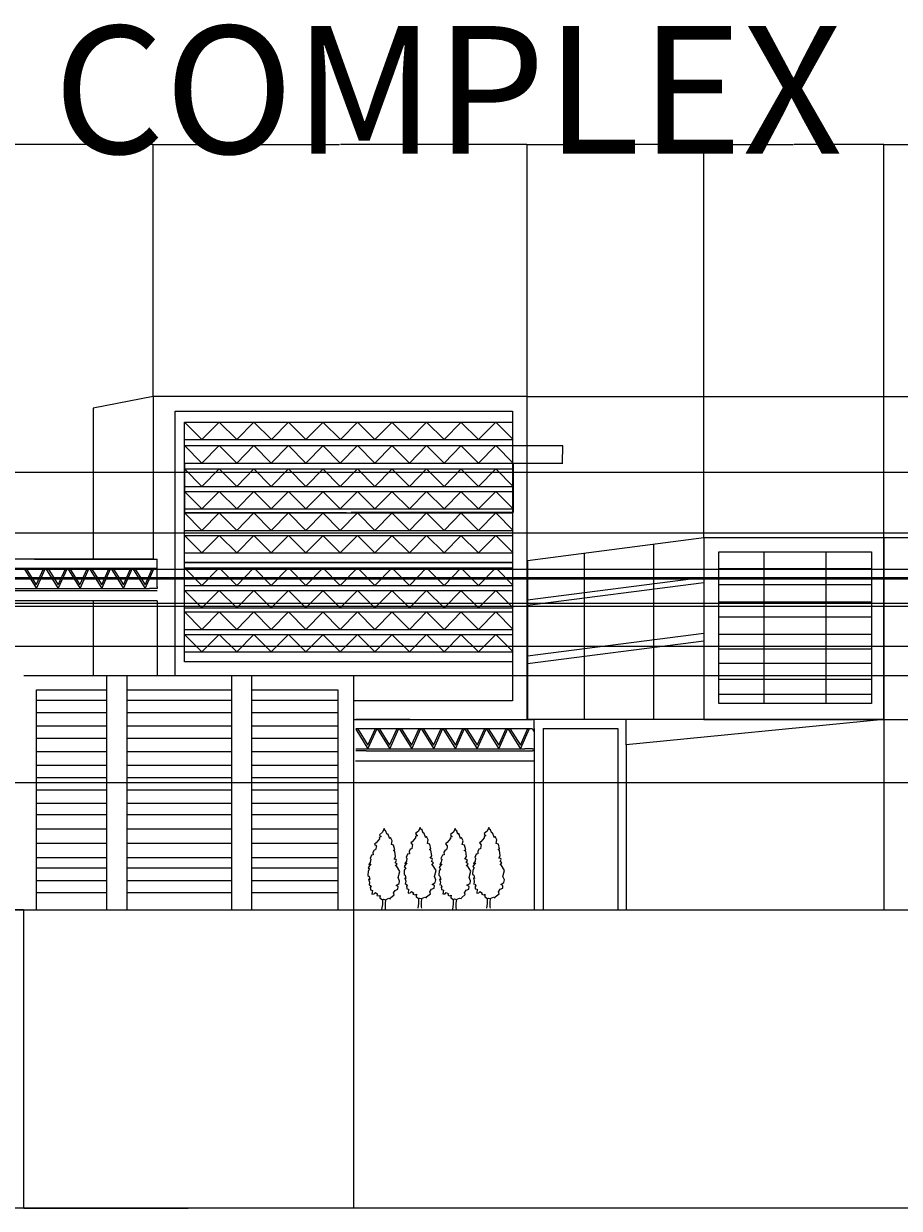
# Model space of a CAD drawing. Units: inches. Extents: x -2248 to 2617, y -128 to 922.
# Tile 6 of 7: x 820 to 1596, y -128 to 922. Entities that reach past the tile are written whole.
import ezdxf

# ---------------------------------------------------------------- set-up
doc = ezdxf.new("R2010")
doc.units = ezdxf.units.IN
doc.header["$MEASUREMENT"] = 0
for name, color, linetype, lineweight in [('A-ANNO-DIMS', 2, 'Continuous', 18), ('A-ANNO-TEXT', 7, 'Continuous', 25), ('A-ELEV', 7, 'Continuous', 25), ('A-ELEV-FACD', 8, 'Continuous', 13), ('L-PLNT', 3, 'Continuous', 18)]:
    doc.layers.add(name, color=color, linetype=linetype, lineweight=lineweight)
doc.styles.get("Standard").update_dxf_attribs({"font": 'arial.ttf'})
doc.dimstyles.get("Standard").update_dxf_attribs({"dimtxt": 0.18, "dimasz": 0.18, "dimexe": 0.18, "dimexo": 0.0625, "dimgap": 0.09, "dimtad": 0, "dimtih": 1, "dimtoh": 1, "dimdec": 4, "dimzin": 0, "dimdsep": 46, "dimtxsty": 'Standard', "dimcen": 0.09, "dimadec": 0, "dimazin": 0, "dimtfac": 1, "dimtdec": 4, "dimtofl": 0, "dimtmove": 0, "dimatfit": 3, "dimfxl": 1, "dimtolj": 1, "dimtzin": 0, "dimarcsym": 0})

# ---------------------------------------------------------------- blocks, each defined once
blk = doc.blocks.new('*U3')
blk.add_lwpolyline([(-2.754, 191.699), (-6.78, 182.851), (-13.682, 176.953), (-11.956, 173.266), (-9.656, 172.529), (-14.257, 170.317), (-13.682, 167.368), (-21.733, 157.783), (-25.184, 154.834), (-21.158, 150.41), (-21.733, 147.461), (-22.884, 140.825), (-26.334, 140.087), (-29.21, 134.926), (-28.635, 129.028), (-32.661, 128.291), (-36.111, 120.18), (-34.386, 118.706), (-35.536, 111.333), (-38.987, 106.171), (-34.386, 107.646), (-40.712, 98.798), (-37.261, 95.849), (-40.712, 90.688), (-41.287, 80.366), (-38.412, 78.154), (-36.686, 70.781), (-39.562, 71.518), (-37.261, 64.145), (-38.412, 57.509), (-36.111, 58.247), (-33.236, 52.348), (-35.536, 53.086), (-34.961, 46.45), (-30.36, 44.975), (-31.51, 36.128), (-26.334, 36.865), (-23.459, 39.814), (-18.283, 36.128), (-20.008, 33.178), (-14.832, 31.704), (-11.956, 33.178), (-12.531, 27.28), (-6.205, 22.856), (-3.905, 24.331), (0.121, 22.856), (8.173, 26.543), (11.624, 25.068), (12.199, 27.28), (21.4, 34.653), (19.675, 39.077), (23.701, 44.975), (30.027, 47.924), (30.602, 53.823), (25.426, 56.772), (32.903, 61.196), (34.053, 67.094), (30.602, 75.205), (34.628, 89.951), (26.576, 103.222), (23.701, 103.222), (28.302, 107.646), (23.701, 110.595), (26.576, 115.756), (25.426, 117.968), (20.825, 118.706), (24.276, 124.604), (22.551, 137.876), (19.1, 139.35), (22.551, 140.825), (19.675, 151.884), (14.499, 153.359), (16.224, 162.207), (12.199, 170.317), (10.473, 167.368), (5.872, 179.165), (4.147, 177.69), (0.696, 187.275), (-0.454, 185.8)], close=True)
for points in [[(-6.813, 23.669), (-6.813, 11.669), (-8.627, 0)], [(0.387, 23.669), (-0.576, 13.271), (-0.576, 3.686), (0, 0)]]:
    blk.add_lwpolyline(points)
blk = doc.blocks.new('FACADE-SCREEN-PANEL')
for p, q in [((0, 15.5), (290.7, 15.5)), ((0, 15.5), (15.6, 0)), ((15.6, 0), (30.8, 15.5)), ((30.8, 15.5), (46.4, 0)), ((46.4, 0), (61.6, 15.5)), ((61.5, 15.5), (77, 0)), ((77, 0), (92.2, 15.5)), ((92.1, 15.5), (107.7, 0)), ((107.7, 0), (122.9, 15.5)), ((122.6, 15.5), (138.1, 0)), ((138.1, 0), (153.4, 15.5)), ((153.2, 15.5), (168.8, 0)), ((168.8, 0), (184, 15.5)), ((183.8, 15.5), (199.3, 0)), ((199.3, 0), (214.5, 15.5)), ((214.4, 15.5), (230, 0)), ((230, 0), (245.2, 15.5)), ((245, 15.5), (260.5, 0)), ((260.5, 0), (275.8, 15.5)), ((275.8, 15.5), (291.3, 0)), ((0, 0), (291.3, 0))]:
    blk.add_line(p, q)
blk = doc.blocks.new('*D10')
at = {"layer": 'A-ANNO-DIMS', "color": 0, "lineweight": -2, "transparency": 16777216}
for p, q in [((962.6, 532.4), (962.6, 488.5)), ((1253.9, 532.4), (1253.9, 488.5)), ((962.8, 488.7), (1106.1, 488.7)), ((1253.7, 488.7), (1110.4, 488.7))]:
    blk.add_line(p, q, dxfattribs=at)
at = {"layer": 'A-ANNO-DIMS', "color": 0, "transparency": 16777216}
for points in [[(962.8, 488.7), (962.8, 488.7), (962.6, 488.7)], [(1253.7, 488.7), (1253.7, 488.7), (1253.9, 488.7)]]:
    blk.add_solid(points, dxfattribs=at)
at = {"layer": 'Defpoints', "color": 0, "transparency": 16777216}
for p in [(962.6, 532.4), (1253.9, 532.4), (1253.9, 488.7)]:
    blk.add_point(p, dxfattribs=at)
at = {"layer": 'A-ANNO-DIMS', "color": 0, "transparency": 16777216, "insert": (1108.3, 488.7), "char_height": 0.18, "attachment_point": 5}
blk.add_mtext('\\A1;FACADE SCREEN PANEL 291 TYP.', dxfattribs=at)
blk = doc.blocks.new('*D11')
at = {"layer": 'A-ANNO-DIMS', "color": 0, "lineweight": -2, "transparency": 16777216}
for p, q in [((1254, 547.9), (1297.8, 547.9)), ((1297.6, 547.7), (1297.6, 540.3)), ((1297.6, 532.6), (1297.6, 540)), ((1254, 532.4), (1297.8, 532.4))]:
    blk.add_line(p, q, dxfattribs=at)
at = {"layer": 'A-ANNO-DIMS', "color": 0, "transparency": 16777216}
for points in [[(1297.6, 547.7), (1297.7, 547.7), (1297.6, 547.9)], [(1297.6, 532.6), (1297.7, 532.6), (1297.6, 532.4)]]:
    blk.add_solid(points, dxfattribs=at)
at = {"layer": 'Defpoints', "color": 0, "transparency": 16777216}
for p in [(1253.9, 547.9), (1297.6, 547.9), (1253.9, 532.4)]:
    blk.add_point(p, dxfattribs=at)
at = {"layer": 'A-ANNO-DIMS', "color": 0, "transparency": 16777216, "insert": (1297.6, 540.1), "char_height": 0.18, "attachment_point": 5}
blk.add_mtext('\\A1;15 TYP.', dxfattribs=at)
blk = doc.blocks.new('*D16')
at = {"layer": 'A-ANNO-DIMS', "color": 0, "lineweight": -2, "transparency": 16777216}
for p, q in [((45.9, 438.4), (2616.5, 438.4)), ((2616.3, 438.3), (2616.3, 287.6)), ((2616.3, 136.6), (2616.3, 287.3)), ((45.9, 136.5), (2616.5, 136.5))]:
    blk.add_line(p, q, dxfattribs=at)
at = {"layer": 'A-ANNO-DIMS', "color": 0, "transparency": 16777216}
for points in [[(2616.2, 438.3), (2616.3, 438.3), (2616.3, 438.4)], [(2616.2, 136.6), (2616.3, 136.6), (2616.3, 136.5)]]:
    blk.add_solid(points, dxfattribs=at)
at = {"layer": 'Defpoints', "color": 0, "transparency": 16777216}
for p in [(45.8, 438.4), (45.8, 136.5), (2616.3, 136.5)]:
    blk.add_point(p, dxfattribs=at)
at = {"layer": 'A-ANNO-DIMS', "color": 0, "transparency": 16777216, "insert": (2616.3, 287.4), "char_height": 0.18, "attachment_point": 5}
blk.add_mtext('\\A1;302', dxfattribs=at)
blk = doc.blocks.new('*D17')
at = {"layer": 'A-ANNO-DIMS', "color": 0, "lineweight": -2, "transparency": 16777216}
for p, q in [((625.1, 524.3), (2616.5, 524.3)), ((2616.3, 524.1), (2616.3, 330.6)), ((2616.3, 136.6), (2616.3, 330.2)), ((553.6, 136.5), (2616.5, 136.5))]:
    blk.add_line(p, q, dxfattribs=at)
at = {"layer": 'A-ANNO-DIMS', "color": 0, "transparency": 16777216}
for points in [[(2616.2, 524.1), (2616.3, 524.1), (2616.3, 524.3)], [(2616.2, 136.6), (2616.3, 136.6), (2616.3, 136.5)]]:
    blk.add_solid(points, dxfattribs=at)
at = {"layer": 'Defpoints', "color": 0, "transparency": 16777216}
for p in [(625.1, 524.3), (553.6, 136.5), (2616.3, 136.5)]:
    blk.add_point(p, dxfattribs=at)
at = {"layer": 'A-ANNO-DIMS', "color": 0, "transparency": 16777216, "insert": (2616.3, 330.4), "char_height": 0.18, "attachment_point": 5}
blk.add_mtext('\\A1;387.9', dxfattribs=at)
blk = doc.blocks.new('*D20')
at = {"layer": 'A-ANNO-DIMS', "color": 0, "lineweight": -2, "transparency": 16777216}
for p, q in [((-1595.3, 429.9), (2616.5, 429.9)), ((2616.3, 429.7), (2616.3, 417.9)), ((2616.3, 405.8), (2616.3, 417.5)), ((-1653.9, 405.6), (2616.5, 405.6))]:
    blk.add_line(p, q, dxfattribs=at)
at = {"layer": 'A-ANNO-DIMS', "color": 0, "transparency": 16777216}
for points in [[(2616.2, 429.7), (2616.3, 429.7), (2616.3, 429.9)], [(2616.2, 405.8), (2616.3, 405.8), (2616.3, 405.6)]]:
    blk.add_solid(points, dxfattribs=at)
at = {"layer": 'Defpoints', "color": 0, "transparency": 16777216}
for p in [(-1595.4, 429.9), (-1654, 405.6), (2616.3, 405.6)]:
    blk.add_point(p, dxfattribs=at)
at = {"layer": 'A-ANNO-DIMS', "color": 0, "transparency": 16777216, "insert": (2616.3, 417.7), "char_height": 0.18, "attachment_point": 5}
blk.add_mtext('\\A1;24.3', dxfattribs=at)
blk = doc.blocks.new('*D21')
at = {"layer": 'A-ANNO-DIMS', "color": 0, "lineweight": -2, "transparency": 16777216}
for p, q in [((-1125.3, 470.6), (2616.5, 470.6)), ((2616.3, 470.4), (2616.3, 451)), ((2616.3, 431.1), (2616.3, 450.6)), ((-1257.9, 430.9), (2616.5, 430.9))]:
    blk.add_line(p, q, dxfattribs=at)
at = {"layer": 'A-ANNO-DIMS', "color": 0, "transparency": 16777216}
for points in [[(2616.2, 470.4), (2616.3, 470.4), (2616.3, 470.6)], [(2616.2, 431.1), (2616.3, 431.1), (2616.3, 430.9)]]:
    blk.add_solid(points, dxfattribs=at)
at = {"layer": 'Defpoints', "color": 0, "transparency": 16777216}
for p in [(-1125.4, 470.6), (-1258, 430.9), (2616.3, 430.9)]:
    blk.add_point(p, dxfattribs=at)
at = {"layer": 'A-ANNO-DIMS', "color": 0, "transparency": 16777216, "insert": (2616.3, 450.8), "char_height": 0.18, "attachment_point": 5}
blk.add_mtext('\\A1;39.705', dxfattribs=at)
blk = doc.blocks.new('*D22')
at = {"layer": 'A-ANNO-DIMS', "color": 0, "lineweight": -2, "transparency": 16777216}
for p, q in [((-733.3, 408.4), (2616.5, 408.4)), ((2616.3, 408.2), (2616.3, 329.1)), ((2616.3, 249.6), (2616.3, 328.7)), ((-719.1, 249.4), (2616.5, 249.4))]:
    blk.add_line(p, q, dxfattribs=at)
at = {"layer": 'A-ANNO-DIMS', "color": 0, "transparency": 16777216}
for points in [[(2616.2, 408.2), (2616.3, 408.2), (2616.3, 408.4)], [(2616.2, 249.6), (2616.3, 249.6), (2616.3, 249.4)]]:
    blk.add_solid(points, dxfattribs=at)
at = {"layer": 'Defpoints', "color": 0, "transparency": 16777216}
for p in [(-733.4, 408.4), (-719.2, 249.4), (2616.3, 249.4)]:
    blk.add_point(p, dxfattribs=at)
at = {"layer": 'A-ANNO-DIMS', "color": 0, "transparency": 16777216, "insert": (2616.3, 328.9), "char_height": 0.18, "attachment_point": 5}
blk.add_mtext('\\A1;159.02', dxfattribs=at)
blk = doc.blocks.new('*D23')
at = {"layer": 'A-ANNO-DIMS', "color": 0, "lineweight": -2, "transparency": 16777216}
for p, q in [((-719.1, 249.4), (2616.5, 249.4)), ((2616.3, 249.2), (2616.3, 193.1)), ((2616.3, 136.6), (2616.3, 192.7)), ((-719.1, 136.5), (2616.5, 136.5))]:
    blk.add_line(p, q, dxfattribs=at)
at = {"layer": 'A-ANNO-DIMS', "color": 0, "transparency": 16777216}
for points in [[(2616.2, 249.2), (2616.3, 249.2), (2616.3, 249.4)], [(2616.2, 136.6), (2616.3, 136.6), (2616.3, 136.5)]]:
    blk.add_solid(points, dxfattribs=at)
at = {"layer": 'Defpoints', "color": 0, "transparency": 16777216}
for p in [(-719.2, 249.4), (-719.2, 136.5), (2616.3, 136.5)]:
    blk.add_point(p, dxfattribs=at)
at = {"layer": 'A-ANNO-DIMS', "color": 0, "transparency": 16777216, "insert": (2616.3, 192.9), "char_height": 0.18, "attachment_point": 5}
blk.add_mtext('\\A1;112.94', dxfattribs=at)
blk = doc.blocks.new('*D24')
at = {"layer": 'A-ANNO-DIMS', "color": 0, "lineweight": -2, "transparency": 16777216}
for p, q in [((-316.1, 370.3), (2616.5, 370.3)), ((2616.3, 370.1), (2616.3, 253.6)), ((2616.3, 136.6), (2616.3, 253.2)), ((-159.8, 136.5), (2616.5, 136.5))]:
    blk.add_line(p, q, dxfattribs=at)
at = {"layer": 'A-ANNO-DIMS', "color": 0, "transparency": 16777216}
for points in [[(2616.2, 370.1), (2616.3, 370.1), (2616.3, 370.3)], [(2616.2, 136.6), (2616.3, 136.6), (2616.3, 136.5)]]:
    blk.add_solid(points, dxfattribs=at)
at = {"layer": 'Defpoints', "color": 0, "transparency": 16777216}
for p in [(-316.2, 370.3), (-159.9, 136.5), (2616.3, 136.5)]:
    blk.add_point(p, dxfattribs=at)
at = {"layer": 'A-ANNO-DIMS', "color": 0, "transparency": 16777216, "insert": (2616.3, 253.4), "char_height": 0.18, "attachment_point": 5}
blk.add_mtext('\\A1;233.87', dxfattribs=at)
blk = doc.blocks.new('*D25')
at = {"layer": 'A-ANNO-DIMS', "color": 0, "lineweight": -2, "transparency": 16777216}
for p, q in [((1112.5, 344.2), (2616.5, 344.2)), ((2616.3, 344), (2616.3, 240.5)), ((2616.3, 136.6), (2616.3, 240.2)), ((1112.5, 136.5), (2616.5, 136.5))]:
    blk.add_line(p, q, dxfattribs=at)
at = {"layer": 'A-ANNO-DIMS', "color": 0, "transparency": 16777216}
for points in [[(2616.2, 344), (2616.3, 344), (2616.3, 344.2)], [(2616.2, 136.6), (2616.3, 136.6), (2616.3, 136.5)]]:
    blk.add_solid(points, dxfattribs=at)
at = {"layer": 'Defpoints', "color": 0, "transparency": 16777216}
for p in [(1112.5, 344.2), (1112.5, 136.5), (2616.3, 136.5)]:
    blk.add_point(p, dxfattribs=at)
at = {"layer": 'A-ANNO-DIMS', "color": 0, "transparency": 16777216, "insert": (2616.3, 240.3), "char_height": 0.18, "attachment_point": 5}
blk.add_mtext('\\A1;207.78', dxfattribs=at)
blk = doc.blocks.new('*D26')
at = {"layer": 'A-ANNO-DIMS', "color": 0, "lineweight": -2, "transparency": 16777216}
for p, q in [((1582.3, 466.3), (2616.5, 466.3)), ((2616.3, 466.1), (2616.3, 385.9)), ((2616.3, 305.4), (2616.3, 385.6)), ((1582.3, 305.2), (2616.5, 305.2))]:
    blk.add_line(p, q, dxfattribs=at)
at = {"layer": 'A-ANNO-DIMS', "color": 0, "transparency": 16777216}
for points in [[(2616.2, 466.1), (2616.3, 466.1), (2616.3, 466.3)], [(2616.2, 305.4), (2616.3, 305.4), (2616.3, 305.2)]]:
    blk.add_solid(points, dxfattribs=at)
at = {"layer": 'Defpoints', "color": 0, "transparency": 16777216}
for p in [(1582.2, 466.3), (1582.2, 305.2), (2616.3, 305.2)]:
    blk.add_point(p, dxfattribs=at)
at = {"layer": 'A-ANNO-DIMS', "color": 0, "transparency": 16777216, "insert": (2616.3, 385.8), "char_height": 0.18, "attachment_point": 5}
blk.add_mtext('\\A1;161.04', dxfattribs=at)
blk = doc.blocks.new('*D28')
at = {"layer": 'A-ANNO-DIMS', "color": 0, "lineweight": -2, "transparency": 16777216}
for p, q in [((1266.1, 591.3), (2616.5, 591.3)), ((2616.3, 591.1), (2616.3, 364)), ((2616.3, 136.6), (2616.3, 363.7)), ((2058.4, 136.5), (2616.5, 136.5))]:
    blk.add_line(p, q, dxfattribs=at)
at = {"layer": 'A-ANNO-DIMS', "color": 0, "transparency": 16777216}
for points in [[(2616.2, 591.1), (2616.3, 591.1), (2616.3, 591.3)], [(2616.2, 136.6), (2616.3, 136.6), (2616.3, 136.5)]]:
    blk.add_solid(points, dxfattribs=at)
at = {"layer": 'Defpoints', "color": 0, "transparency": 16777216}
for p in [(1266.1, 591.3), (2616.3, 591.3), (2058.4, 136.5)]:
    blk.add_point(p, dxfattribs=at)
at = {"layer": 'A-ANNO-DIMS', "color": 0, "transparency": 16777216, "insert": (2616.3, 363.9), "char_height": 0.18, "attachment_point": 5}
blk.add_mtext('\\A1;454.8', dxfattribs=at)
blk = doc.blocks.new('*D31')
at = {"layer": 'A-ANNO-DIMS', "color": 0, "lineweight": -2, "transparency": 16777216}
for p, q in [((934.8, 447.2), (-2247.7, 447.2)), ((-2247.5, 447), (-2247.5, 292)), ((-2247.5, 136.6), (-2247.5, 291.6)), ((820, 136.5), (-2247.7, 136.5))]:
    blk.add_line(p, q, dxfattribs=at)
at = {"layer": 'A-ANNO-DIMS', "color": 0, "transparency": 16777216}
for points in [[(-2247.5, 447), (-2247.5, 447), (-2247.5, 447.2)], [(-2247.5, 136.6), (-2247.5, 136.6), (-2247.5, 136.5)]]:
    blk.add_solid(points, dxfattribs=at)
at = {"layer": 'Defpoints', "color": 0, "transparency": 16777216}
for p in [(934.9, 447.2), (-2247.5, 136.5), (820.1, 136.5)]:
    blk.add_point(p, dxfattribs=at)
at = {"layer": 'A-ANNO-DIMS', "color": 0, "transparency": 16777216, "insert": (-2247.5, 291.8), "char_height": 0.18, "attachment_point": 5}
blk.add_mtext('\\A1;310.7', dxfattribs=at)
blk = doc.blocks.new('*D33')
at = {"layer": 'A-ANNO-DIMS', "color": 0, "lineweight": -2, "transparency": 16777216}
for p, q in [((2393, 136.4), (2393, -127.9)), ((-2024.3, 122), (-2024.3, -127.9)), ((-2024.1, -127.7), (184, -127.7)), ((2392.8, -127.7), (184.7, -127.7))]:
    blk.add_line(p, q, dxfattribs=at)
at = {"layer": 'A-ANNO-DIMS', "color": 0, "transparency": 16777216}
for points in [[(-2024.1, -127.6), (-2024.1, -127.7), (-2024.3, -127.7)], [(2392.8, -127.6), (2392.8, -127.7), (2393, -127.7)]]:
    blk.add_solid(points, dxfattribs=at)
at = {"layer": 'Defpoints', "color": 0, "transparency": 16777216}
for p in [(2393, 136.5), (-2024.3, 122.1), (2393, -127.7)]:
    blk.add_point(p, dxfattribs=at)
at = {"layer": 'A-ANNO-DIMS', "color": 0, "transparency": 16777216, "insert": (184.4, -127.7), "char_height": 0.18, "attachment_point": 5}
blk.add_mtext('\\A1;4417', dxfattribs=at)
blk = doc.blocks.new('*D50')
at = {"layer": 'A-ANNO-DIMS', "color": 0, "lineweight": -2, "transparency": 16777216}
for p, q in [((625.1, 524.4), (625.1, 814.7)), ((625.2, 814.5), (779.6, 814.5)), ((934.7, 814.5), (780.4, 814.5)), ((934.9, 591.3), (934.9, 814.7))]:
    blk.add_line(p, q, dxfattribs=at)
at = {"layer": 'A-ANNO-DIMS', "color": 0, "transparency": 16777216}
for points in [[(625.2, 814.5), (625.2, 814.5), (625.1, 814.5)], [(934.7, 814.5), (934.7, 814.5), (934.9, 814.5)]]:
    blk.add_solid(points, dxfattribs=at)
at = {"layer": 'Defpoints', "color": 0, "transparency": 16777216}
for p in [(934.9, 814.5), (934.9, 591.3), (625.1, 524.3)]:
    blk.add_point(p, dxfattribs=at)
at = {"layer": 'A-ANNO-DIMS', "color": 0, "transparency": 16777216, "insert": (780, 814.5), "char_height": 0.18, "attachment_point": 5}
blk.add_mtext('\\A1;309.8', dxfattribs=at)
blk = doc.blocks.new('*D51')
at = {"layer": 'A-ANNO-DIMS', "color": 0, "lineweight": -2, "transparency": 16777216}
for p, q in [((934.9, 591.3), (934.9, 814.7)), ((935, 814.5), (1100.1, 814.5)), ((1265.9, 814.5), (1100.9, 814.5)), ((1266.1, 591.3), (1266.1, 814.7))]:
    blk.add_line(p, q, dxfattribs=at)
at = {"layer": 'A-ANNO-DIMS', "color": 0, "transparency": 16777216}
for points in [[(935, 814.5), (935, 814.5), (934.9, 814.5)], [(1265.9, 814.5), (1265.9, 814.5), (1266.1, 814.5)]]:
    blk.add_solid(points, dxfattribs=at)
at = {"layer": 'Defpoints', "color": 0, "transparency": 16777216}
for p in [(1266.1, 814.5), (934.9, 591.3), (1266.1, 591.3)]:
    blk.add_point(p, dxfattribs=at)
at = {"layer": 'A-ANNO-DIMS', "color": 0, "transparency": 16777216, "insert": (1100.5, 814.5), "char_height": 0.18, "attachment_point": 5}
blk.add_mtext('\\A1;331.2', dxfattribs=at)
blk = doc.blocks.new('*D52')
at = {"layer": 'A-ANNO-DIMS', "color": 0, "lineweight": -2, "transparency": 16777216}
for p, q in [((1266.1, 591.3), (1266.1, 814.7)), ((1266.3, 814.5), (1343.9, 814.5)), ((1422.5, 814.5), (1344.8, 814.5)), ((1422.7, 466.3), (1422.7, 814.7))]:
    blk.add_line(p, q, dxfattribs=at)
at = {"layer": 'A-ANNO-DIMS', "color": 0, "transparency": 16777216}
for points in [[(1266.3, 814.5), (1266.3, 814.5), (1266.1, 814.5)], [(1422.5, 814.5), (1422.5, 814.5), (1422.7, 814.5)]]:
    blk.add_solid(points, dxfattribs=at)
at = {"layer": 'Defpoints', "color": 0, "transparency": 16777216}
for p in [(1422.7, 814.5), (1266.1, 591.3), (1422.7, 466.3)]:
    blk.add_point(p, dxfattribs=at)
at = {"layer": 'A-ANNO-DIMS', "color": 0, "transparency": 16777216, "insert": (1344.4, 814.5), "char_height": 0.18, "attachment_point": 5}
blk.add_mtext('\\A1;156.62', dxfattribs=at)
blk = doc.blocks.new('*D53')
at = {"layer": 'A-ANNO-DIMS', "color": 0, "lineweight": -2, "transparency": 16777216}
for p, q in [((1422.7, 466.3), (1422.7, 814.7)), ((1422.9, 814.5), (1502.1, 814.5)), ((1582, 814.5), (1502.8, 814.5)), ((1582.2, 466.3), (1582.2, 814.7))]:
    blk.add_line(p, q, dxfattribs=at)
at = {"layer": 'A-ANNO-DIMS', "color": 0, "transparency": 16777216}
for points in [[(1422.9, 814.5), (1422.9, 814.5), (1422.7, 814.5)], [(1582, 814.5), (1582, 814.5), (1582.2, 814.5)]]:
    blk.add_solid(points, dxfattribs=at)
at = {"layer": 'Defpoints', "color": 0, "transparency": 16777216}
for p in [(1582.2, 814.5), (1422.7, 466.3), (1582.2, 466.3)]:
    blk.add_point(p, dxfattribs=at)
at = {"layer": 'A-ANNO-DIMS', "color": 0, "transparency": 16777216, "insert": (1502.5, 814.5), "char_height": 0.18, "attachment_point": 5}
blk.add_mtext('\\A1;159.5', dxfattribs=at)
blk = doc.blocks.new('*D54')
at = {"layer": 'A-ANNO-DIMS', "color": 0, "lineweight": -2, "transparency": 16777216}
for p, q in [((1582.2, 305.3), (1582.2, 814.7)), ((1582.4, 814.5), (1819.8, 814.5)), ((2058.2, 814.5), (1820.7, 814.5)), ((2058.4, 305.3), (2058.4, 814.7))]:
    blk.add_line(p, q, dxfattribs=at)
at = {"layer": 'A-ANNO-DIMS', "color": 0, "transparency": 16777216}
for points in [[(1582.4, 814.5), (1582.4, 814.5), (1582.2, 814.5)], [(2058.2, 814.5), (2058.2, 814.5), (2058.4, 814.5)]]:
    blk.add_solid(points, dxfattribs=at)
at = {"layer": 'Defpoints', "color": 0, "transparency": 16777216}
for p in [(2058.4, 814.5), (1582.2, 305.2), (2058.4, 305.2)]:
    blk.add_point(p, dxfattribs=at)
at = {"layer": 'A-ANNO-DIMS', "color": 0, "transparency": 16777216, "insert": (1820.3, 814.5), "char_height": 0.18, "attachment_point": 5}
blk.add_mtext('\\A1;476.15', dxfattribs=at)
blk = doc.blocks.new('*D57')
at = {"layer": 'A-ANNO-DIMS', "color": 0, "lineweight": -2, "transparency": 16777216}
for p, q in [((820.1, 136.4), (820.1, -127.9)), ((1112.5, 136.4), (1112.5, -127.9)), ((820.3, -127.7), (965.9, -127.7)), ((1112.3, -127.7), (966.7, -127.7))]:
    blk.add_line(p, q, dxfattribs=at)
at = {"layer": 'A-ANNO-DIMS', "color": 0, "transparency": 16777216}
for points in [[(820.3, -127.6), (820.3, -127.7), (820.1, -127.7)], [(1112.3, -127.6), (1112.3, -127.7), (1112.5, -127.7)]]:
    blk.add_solid(points, dxfattribs=at)
at = {"layer": 'Defpoints', "color": 0, "transparency": 16777216}
for p in [(820.1, 136.5), (1112.5, 136.5), (1112.5, -127.7)]:
    blk.add_point(p, dxfattribs=at)
at = {"layer": 'A-ANNO-DIMS', "color": 0, "transparency": 16777216, "insert": (966.3, -127.7), "char_height": 0.18, "attachment_point": 5}
blk.add_mtext('\\A1;292.4', dxfattribs=at)

msp = doc.modelspace()

# ---------------------------------------------------------------- linework, layer by layer
at = {"layer": 'A-ELEV'}
for p, q in [((934.8599, 591.2689), (881.9153, 581.0202)), ((1266.0706, 591.2689), (934.8599, 591.2689)), ((934.8599, 591.2689), (934.8599, 447.1806)), ((1266.0706, 305.2491), (1266.0706, 591.2689)), ((881.9153, 581.0202), (881.9153, 447.1785)), ((954.5101, 578.2931), (1253.2702, 578.2931)), ((954.5101, 344.2299), (954.5101, 578.2931)), ((1253.2702, 578.2931), (1253.2702, 321.5917)), ((962.601, 568.6073), (1253.2702, 568.6073)), ((962.601, 356.3956), (962.601, 568.6073)), ((962.601, 568.6073), (978.1733, 553.154)), ((978.1733, 553.154), (993.3817, 568.6073)), ((993.3845, 568.6073), (1008.9567, 553.154)), ((1008.9567, 553.154), (1024.1652, 568.6073)), ((1024.0616, 568.6073), (1039.6339, 553.154)), ((1039.6339, 553.154), (1054.8423, 568.6073)), ((1054.6964, 568.6073), (1070.2686, 553.154)), ((1070.2686, 553.154), (1085.477, 568.6073)), ((1085.1738, 568.6073), (1100.746, 553.154)), ((1100.746, 553.154), (1115.9544, 568.6073)), ((1115.8362, 568.6073), (1131.4084, 553.154)), ((1131.4084, 553.154), (1146.6169, 568.6073)), ((1146.3674, 568.6073), (1161.9396, 553.154)), ((1161.9396, 553.154), (1177.1481, 568.6073)), ((1177.0447, 568.6073), (1192.617, 553.154)), ((1192.617, 553.154), (1207.8254, 568.6073)), ((1207.576, 568.6073), (1223.1482, 553.154)), ((1223.1482, 553.154), (1238.3566, 568.6073)), ((1238.351, 568.6073), (1253.9233, 553.154)), ((962.601, 553.154), (1253.9233, 553.154)), ((1266.5247, 446.1129), (1422.6951, 466.287)), ((1422.6951, 466.287), (1422.6951, 305.2491)), ((1422.6951, 466.287), (1582.2049, 466.287)), ((1582.2049, 466.287), (1582.2049, 305.2491)), ((1316.8274, 452.611), (1316.8274, 305.2491)), ((1377.9797, 460.5106), (1377.9797, 305.2491)), ((1435.9942, 453.6809), (1571.2541, 453.6809)), ((1436.0053, 319.2369), (1436.0053, 453.6809)), ((1476.1529, 319.2369), (1476.1529, 453.6809)), ((1531.177, 319.2369), (1531.177, 453.6809)), ((1571.2541, 453.6809), (1571.2541, 319.2369)), ((829.7811, 447.1806), (781.9719, 447.1806)), ((829.7811, 447.1806), (938.3811, 447.1806)), ((934.8599, 447.1806), (938.3811, 447.1806)), ((938.3811, 422.7386), (938.3811, 447.1806)), ((962.601, 444.7115), (1253.9233, 444.7115)), ((1253.2702, 444.0968), (962.601, 444.0968)), ((1266.5247, 446.1129), (1266.5247, 305.2491)), ((781.9719, 439.2108), (938.3811, 439.2108)), ((820.2985, 439.2108), (831.5025, 421.2778)), ((822.1385, 439.2051), (831.4178, 424.3527)), ((831.4178, 424.3527), (838.1304, 439.2108)), ((831.5025, 421.2778), (839.6036, 439.2094)), ((839.7182, 439.2108), (850.9222, 421.2778)), ((841.5581, 439.2051), (850.8375, 424.3527)), ((850.8375, 424.3527), (857.5501, 439.2108)), ((850.9222, 421.2778), (859.0233, 439.2094)), ((859.0051, 439.2108), (870.2091, 421.2778)), ((860.8451, 439.2051), (870.1244, 424.3527)), ((870.1244, 424.3527), (876.837, 439.2108)), ((870.2091, 421.2778), (878.3102, 439.2094)), ((878.292, 439.2108), (889.496, 421.2778)), ((880.132, 439.2051), (889.4113, 424.3527)), ((889.4113, 424.3527), (896.1239, 439.2108)), ((889.496, 421.2778), (897.5971, 439.2094)), ((897.4316, 439.2108), (908.6357, 421.2778)), ((899.2716, 439.2051), (908.551, 424.3527)), ((908.551, 424.3527), (915.2636, 439.2108)), ((908.6357, 421.2778), (916.7368, 439.2094)), ((916.6236, 439.2108), (927.8276, 421.2778)), ((918.4635, 439.2051), (927.7429, 424.3527)), ((927.7429, 424.3527), (934.4555, 439.2108)), ((927.8276, 421.2778), (935.9287, 439.2094)), ((1266.5247, 411.0642), (1422.6951, 431.2383)), ((1436.0053, 438.8687), (1571.2541, 438.8687)), ((781.9719, 421.26), (930.0437, 421.26)), ((887.0665, 421.26), (887.0814, 421.2274)), ((887.0814, 421.2274), (887.0994, 421.26)), ((930.0437, 421.26), (931.6985, 421.26)), ((938.3811, 421.26), (931.6985, 421.26)), ((938.3811, 422.7386), (938.3811, 421.26)), ((1266.5247, 406.4352), (1422.6951, 426.6092)), ((1436.0053, 424.7671), (1571.2541, 424.7671)), ((938.3811, 410.2355), (625.2262, 410.2355)), ((791.2768, 419.5059), (918.2951, 419.5059)), ((881.9153, 410.2355), (881.9153, 344.2299)), ((918.2951, 419.5059), (930.0437, 419.5059)), ((930.0437, 419.5059), (938.3811, 419.5059)), ((938.3811, 410.2355), (938.3599, 344.2299)), ((1436.0053, 409.4212), (1571.2541, 409.4212)), ((1436.0053, 396.149), (1571.2541, 396.149)), ((1266.5247, 361.467), (1422.6951, 381.6411)), ((1436.0053, 380.8031), (1571.2541, 380.8031)), ((1266.5247, 354.8541), (1422.6951, 375.0281)), ((1436.0053, 367.8338), (1571.2541, 367.8338)), ((1253.2702, 356.3956), (962.601, 356.3956)), ((1436.0053, 354.9764), (1571.2541, 354.9764)), ((820.2683, 344.2299), (894.0201, 344.2299)), ((894.0201, 136.4519), (894.0201, 344.2299)), ((894.0201, 344.2299), (911.5297, 344.2299)), ((911.5297, 344.2299), (911.5297, 136.4519)), ((911.5297, 344.2299), (1112.486, 344.2299)), ((1004.6069, 136.4519), (1004.6069, 344.2299)), ((1022.1164, 344.2299), (1022.1164, 136.4519)), ((1112.486, 344.2299), (1112.486, 136.4519)), ((1436.0053, 340.8747), (1571.2541, 340.8747)), ((831.6824, 136.4519), (831.6824, 331.3761)), ((831.6824, 331.3761), (894.0201, 331.3761)), ((911.5297, 331.3761), (1004.6069, 331.3761)), ((1022.1164, 331.3761), (1098.4389, 331.3761)), ((1098.4389, 331.3761), (1098.4389, 136.4519)), ((1436.0053, 327.6026), (1571.2541, 327.6026)), ((831.6824, 322.2649), (894.0201, 322.2649)), ((911.5297, 322.2649), (1004.6069, 322.2649)), ((1022.1164, 322.2649), (1098.4389, 322.2649)), ((1253.2702, 321.5917), (1112.486, 321.5917)), ((1571.2541, 319.2369), (1436.0053, 319.2369)), ((831.6824, 311.3314), (894.0201, 311.3314)), ((911.5297, 311.3314), (1004.6069, 311.3314)), ((1022.1164, 311.3314), (1098.4389, 311.3314)), ((1112.486, 305.2491), (1266.0706, 305.2491)), ((1162.2639, 305.2491), (1114.4547, 305.2491)), ((1162.2639, 305.2491), (1270.864, 305.2491)), ((1422.6951, 305.2491), (1266.5247, 305.2491)), ((1267.3428, 305.2491), (1270.864, 305.2491)), ((1309.3084, 305.2491), (1270.9782, 305.2491)), ((1272.3912, 297.2736), (1272.3912, 305.2491)), ((1582.2049, 305.2491), (1353.9083, 282.6642)), ((1353.9083, 282.6642), (1353.9083, 305.2491)), ((1582.2049, 305.2491), (1422.6951, 305.2491)), ((1422.6951, 305.2491), (2058.3545, 305.2491)), ((1582.2049, 305.2491), (1582.2049, 136.4519)), ((831.6824, 299.4868), (894.0201, 299.4868)), ((911.5297, 299.4868), (1004.6069, 299.4868)), ((1022.1164, 299.4868), (1098.4389, 299.4868)), ((1114.4547, 297.2793), (1270.864, 297.2793)), ((1114.4547, 296.5958), (1125.2318, 279.3462)), ((1115.8677, 297.2736), (1125.1471, 282.4211)), ((1125.1471, 282.4211), (1131.8596, 297.2793)), ((1125.2318, 279.3462), (1133.3329, 297.2779)), ((1133.3044, 297.2793), (1144.5084, 279.3462)), ((1135.1444, 297.2736), (1144.4237, 282.4211)), ((1144.4237, 282.4211), (1151.1363, 297.2793)), ((1144.5084, 279.3462), (1152.6095, 297.2779)), ((1152.7813, 297.2793), (1163.9853, 279.3462)), ((1154.6213, 297.2736), (1163.9007, 282.4211)), ((1163.9007, 282.4211), (1170.6132, 297.2793)), ((1163.9853, 279.3462), (1172.0865, 297.2779)), ((1172.201, 297.2793), (1183.405, 279.3462)), ((1174.041, 297.2736), (1183.3203, 282.4211)), ((1183.3203, 282.4211), (1190.0329, 297.2793)), ((1183.405, 279.3462), (1191.5061, 297.2779)), ((1191.4879, 297.2793), (1202.6919, 279.3462)), ((1193.3279, 297.2736), (1202.6072, 282.4211)), ((1202.6072, 282.4211), (1209.3198, 297.2793)), ((1202.6919, 279.3462), (1210.793, 297.2779)), ((1210.7748, 297.2793), (1221.9788, 279.3462)), ((1212.6148, 297.2736), (1221.8941, 282.4211)), ((1221.8941, 282.4211), (1228.6067, 297.2793)), ((1221.9788, 279.3462), (1230.08, 297.2779)), ((1229.9145, 297.2793), (1241.1185, 279.3462)), ((1231.7544, 297.2736), (1241.0338, 282.4211)), ((1241.0338, 282.4211), (1247.7464, 297.2793)), ((1241.1185, 279.3462), (1249.2196, 297.2779)), ((1249.1064, 297.2793), (1260.3104, 279.3462)), ((1250.7149, 297.2793), (1250.7184, 297.2736)), ((1250.9463, 297.2736), (1260.2257, 282.4211)), ((1260.2257, 282.4211), (1266.9383, 297.2793)), ((1260.3104, 279.3462), (1268.4115, 297.2779)), ((1270.9782, 296.5958), (1272.3912, 294.3342)), ((1272.3912, 297.2736), (1272.3912, 136.4519)), ((1280.2557, 297.2736), (1280.2557, 136.4519)), ((1280.2557, 297.2736), (1346.4488, 297.2736)), ((1289.8448, 297.2522), (1289.8564, 297.2779)), ((1346.4488, 297.2736), (1346.4488, 136.4519)), ((831.6824, 288.5534), (894.0201, 288.5534)), ((911.5297, 288.5534), (1004.6069, 288.5534)), ((1022.1164, 288.5534), (1098.4389, 288.5534)), ((831.6824, 276.7088), (894.0201, 276.7088)), ((911.5297, 276.7088), (1004.6069, 276.7088)), ((1022.1164, 276.7088), (1098.4389, 276.7088)), ((1114.4547, 279.3285), (1262.5265, 279.3285)), ((1123.7597, 277.5744), (1114.4547, 277.5744)), ((1123.7597, 277.5744), (1250.7779, 277.5744)), ((1219.5494, 279.3285), (1219.5643, 279.2958)), ((1219.5643, 279.2958), (1219.5822, 279.3285)), ((1250.7779, 277.5744), (1262.5265, 277.5744)), ((1262.5265, 279.3285), (1264.1813, 279.3285)), ((1262.5265, 277.5744), (1270.864, 277.5744)), ((1270.864, 279.3285), (1264.1813, 279.3285)), ((1270.9782, 279.3285), (1272.3912, 279.3285)), ((1272.3912, 277.5744), (1270.9782, 277.5744)), ((1353.9083, 282.6642), (1353.9083, 136.4519)), ((831.6824, 264.8642), (894.0201, 264.8642)), ((911.5297, 264.8642), (1004.6069, 264.8642)), ((1022.1164, 264.8642), (1098.4389, 264.8642)), ((1272.3912, 268.3039), (1114.2325, 268.3039)), ((831.6824, 253.9307), (894.0201, 253.9307)), ((911.5297, 253.9307), (1004.6069, 253.9307)), ((1022.1164, 253.9307), (1098.4389, 253.9307)), ((831.6824, 242.9972), (894.0201, 242.9972)), ((911.5297, 242.9972), (1004.6069, 242.9972)), ((1022.1164, 242.9972), (1098.4389, 242.9972)), ((831.6824, 231.1527), (894.0201, 231.1527)), ((911.5297, 231.1527), (1004.6069, 231.1527)), ((1022.1164, 231.1527), (1098.4389, 231.1527)), ((831.6824, 221.1303), (894.0201, 221.1303)), ((911.5297, 221.1303), (1004.6069, 221.1303)), ((1022.1164, 221.1303), (1098.4389, 221.1303)), ((831.6824, 208.3746), (894.0201, 208.3746)), ((911.5297, 208.3746), (1004.6069, 208.3746)), ((1022.1164, 208.3746), (1098.4389, 208.3746)), ((831.6824, 195.6189), (894.0201, 195.6189)), ((911.5297, 195.6189), (1004.6069, 195.6189)), ((1022.1164, 195.6189), (1098.4389, 195.6189)), ((831.6824, 182.8632), (894.0201, 182.8632)), ((911.5297, 182.8632), (1004.6069, 182.8632)), ((1022.1164, 182.8632), (1098.4389, 182.8632)), ((831.6824, 173.7519), (894.0201, 173.7519)), ((911.5297, 173.7519), (1004.6069, 173.7519)), ((1022.1164, 173.7519), (1098.4389, 173.7519)), ((831.6824, 162.5788), (894.0201, 162.5788)), ((911.5297, 162.5788), (1004.6069, 162.5788)), ((1022.1164, 162.5788), (1098.4389, 162.5788)), ((831.6824, 151.8268), (894.0201, 151.8268)), ((911.5297, 151.8268), (1004.6069, 151.8268)), ((1022.1164, 151.8268), (1098.4389, 151.8268)), ((517.5185, 136.4519), (894.0201, 136.4519)), ((894.0201, 136.4519), (911.5297, 136.4519)), ((911.5297, 136.4519), (1375.9892, 136.4519)), ((1375.9892, 136.4519), (2393.0245, 136.4519))]:
    msp.add_line(p, q, dxfattribs=at)

# ---------------------------------------------------------------- block references
at = {"layer": 'A-ELEV-FACD'}
for p in [(962.601, 532.413), (962.601, 511.6717), (962.601, 491.7769), (962.601, 472.6441), (962.601, 452.7493), (962.601, 423.9705), (962.601, 404.0758), (962.601, 384.9429), (962.601, 365.0482)]:
    msp.add_blockref('FACADE-SCREEN-PANEL', p, dxfattribs=at)
at = {"layer": 'L-PLNT', "xscale": 0.373818396241174, "yscale": 0.373818396241174, "zscale": 0.373818396241174}
for p in [(1140.5459, 136.9852), (1172.567, 137.9288), (1203.3572, 137.1087), (1233.3263, 137.9288)]:
    msp.add_blockref('*U3', p, dxfattribs=at)

# ---------------------------------------------------------------- texts
at = {"layer": 'A-ANNO-TEXT'}
msp.add_text('MEGA   SCALE   INSTITUTIONAL   COMPLEX    ', height=113.064343, dxfattribs=at).set_placement((-1470.2311, 806.5595))

# ---------------------------------------------------------------- dimensions: what is measured, and where the dimension line sits
at = {"layer": 'A-ANNO-DIMS'}
for base, p1, p2, override, picture, middle in [((934.8599, 814.5189), (625.0568, 524.3284), (934.8599, 591.2689), {"dimdec": 1, "dimlfac": 1, "dimrnd": 0, "dimzin": 0, "dimdsep": 46, "dimlunit": 2}, '*D50', (779.9584, 814.5189)), ((1266.0706, 814.5189), (934.8599, 591.2689), (1266.0706, 591.2689), {"dimdec": 1, "dimlfac": 1, "dimrnd": 0, "dimzin": 0, "dimdsep": 46, "dimlunit": 2}, '*D51', (1100.4653, 814.5189)), ((1422.6951, 814.5189), (1266.0706, 591.2689), (1422.6951, 466.287), {"dimdec": 2, "dimlfac": 1, "dimrnd": 0, "dimzin": 0, "dimdsep": 46, "dimlunit": 2}, '*D52', (1344.3829, 814.5189)), ((1582.2049, 814.5189), (1422.6951, 466.287), (1582.2049, 466.287), {"dimdec": 1, "dimlfac": 1, "dimrnd": 0, "dimzin": 0, "dimdsep": 46, "dimlunit": 2}, '*D53', (1502.45, 814.5189)), ((2058.3545, 814.5189), (1582.2049, 305.2491), (2058.3545, 305.2491), {"dimdec": 2, "dimlfac": 1, "dimrnd": 0, "dimzin": 0, "dimdsep": 46, "dimlunit": 2}, '*D54', (1820.2797, 814.5189)), ((2393.0245, -127.6745), (-2024.254, 122.0847), (2393.0245, 136.4519), {"dimdec": 0, "dimlfac": 1, "dimrnd": 0, "dimzin": 0, "dimdsep": 46, "dimlunit": 2}, '*D33', (184.3853, -127.6745)), ((1112.486, -127.6745), (820.0929, 136.4519), (1112.486, 136.4519), {"dimdec": 1, "dimlfac": 1, "dimrnd": 0, "dimzin": 0, "dimdsep": 46, "dimlunit": 2}, '*D57', (966.2895, -127.6745))]:
    dim = msp.add_linear_dim(base=base, p1=p1, p2=p2, dimstyle='Standard', override=override, dxfattribs=at)
    dim.commit()
    dim.dimension.update_dxf_attribs({"geometry": picture, "text_midpoint": middle})
for base, p1, p2, override, picture, middle in [((2616.2745, 591.2689), (2058.3545, 136.4519), (1266.0706, 591.2689), {"dimdec": 1, "dimlfac": 1, "dimrnd": 0, "dimzin": 0, "dimdsep": 46, "dimlunit": 2}, '*D28', (2616.2745, 363.8604)), ((2616.2745, 136.4519), (625.0568, 524.3284), (553.5648, 136.4519), {"dimdec": 1, "dimlfac": 1, "dimrnd": 0, "dimzin": 0, "dimdsep": 46, "dimlunit": 2}, '*D17', (2616.2745, 330.3901)), ((2616.2745, 430.9238), (-1125.4072, 470.6286), (-1257.9572, 430.9238), {"dimdec": 3, "dimlfac": 1, "dimrnd": 0, "dimzin": 0, "dimdsep": 46, "dimlunit": 2}, '*D21', (2616.2745, 450.7762)), ((2616.2745, 305.2491), (1582.2049, 466.287), (1582.2049, 305.2491), {"dimdec": 2, "dimlfac": 1, "dimrnd": 0, "dimzin": 0, "dimdsep": 46, "dimlunit": 2}, '*D26', (2616.2745, 385.768)), ((-2247.504, 136.4519), (934.8599, 447.1806), (820.0929, 136.4519), {"dimdec": 1, "dimlfac": 1, "dimrnd": 0, "dimzin": 0, "dimdsep": 46, "dimlunit": 2}, '*D31', (-2247.504, 291.8162)), ((2616.2745, 136.4519), (45.827, 438.443), (45.827, 136.4519), {"dimdec": 0, "dimlfac": 1, "dimrnd": 0, "dimzin": 0, "dimdsep": 46, "dimlunit": 2}, '*D16', (2616.2745, 287.4474)), ((2616.2745, 405.5754), (-1595.3791, 429.8743), (-1653.9599, 405.5754), {"dimdec": 1, "dimlfac": 1, "dimrnd": 0, "dimzin": 0, "dimdsep": 46, "dimlunit": 2}, '*D20', (2616.2745, 417.7249)), ((2616.2745, 249.389), (-733.3752, 408.4102), (-719.1936, 249.389), {"dimdec": 2, "dimlfac": 1, "dimrnd": 0, "dimzin": 0, "dimdsep": 46, "dimlunit": 2}, '*D22', (2616.2745, 328.8996)), ((2616.2745, 136.4519), (-316.2025, 370.3211), (-159.9067, 136.4519), {"dimdec": 2, "dimlfac": 1, "dimrnd": 0, "dimzin": 0, "dimdsep": 46, "dimlunit": 2}, '*D24', (2616.2745, 253.3865)), ((2616.2745, 136.4519), (1112.486, 344.2299), (1112.486, 136.4519), {"dimdec": 2, "dimlfac": 1, "dimrnd": 0, "dimzin": 0, "dimdsep": 46, "dimlunit": 2}, '*D25', (2616.2745, 240.3409)), ((2616.2745, 136.4519), (-719.1936, 249.389), (-719.1936, 136.4519), {"dimdec": 2, "dimlfac": 1, "dimrnd": 0, "dimzin": 0, "dimdsep": 46, "dimlunit": 2}, '*D23', (2616.2745, 192.9204))]:
    dim = msp.add_linear_dim(base=base, p1=p1, p2=p2, angle=90, dimstyle='Standard', override=override, dxfattribs=at)
    dim.commit()
    dim.dimension.update_dxf_attribs({"geometry": picture, "text_midpoint": middle})
dim = msp.add_linear_dim(base=(1297.6216, 547.8659), p1=(1253.9233, 532.4126), p2=(1253.9233, 547.8659), angle=90, text='<> TYP.', dimstyle='Standard', override={"dimdec": 0, "dimrnd": 0, "dimzin": 0, "dimlunit": 2}, dxfattribs=at)
dim.commit()
dim.dimension.update_dxf_attribs({"geometry": '*D11', "text_midpoint": (1297.6216, 540.1393)})
dim = msp.add_linear_dim(base=(1253.9233, 488.7143), p1=(962.601, 532.4126), p2=(1253.9233, 532.4126), text='FACADE SCREEN PANEL <> TYP.', dimstyle='Standard', override={"dimdec": 0, "dimrnd": 0, "dimzin": 0, "dimlunit": 2}, dxfattribs=at)
dim.commit()
dim.dimension.update_dxf_attribs({"geometry": '*D10', "text_midpoint": (1108.2621, 488.7143)})

doc.saveas('drawing.dxf')
